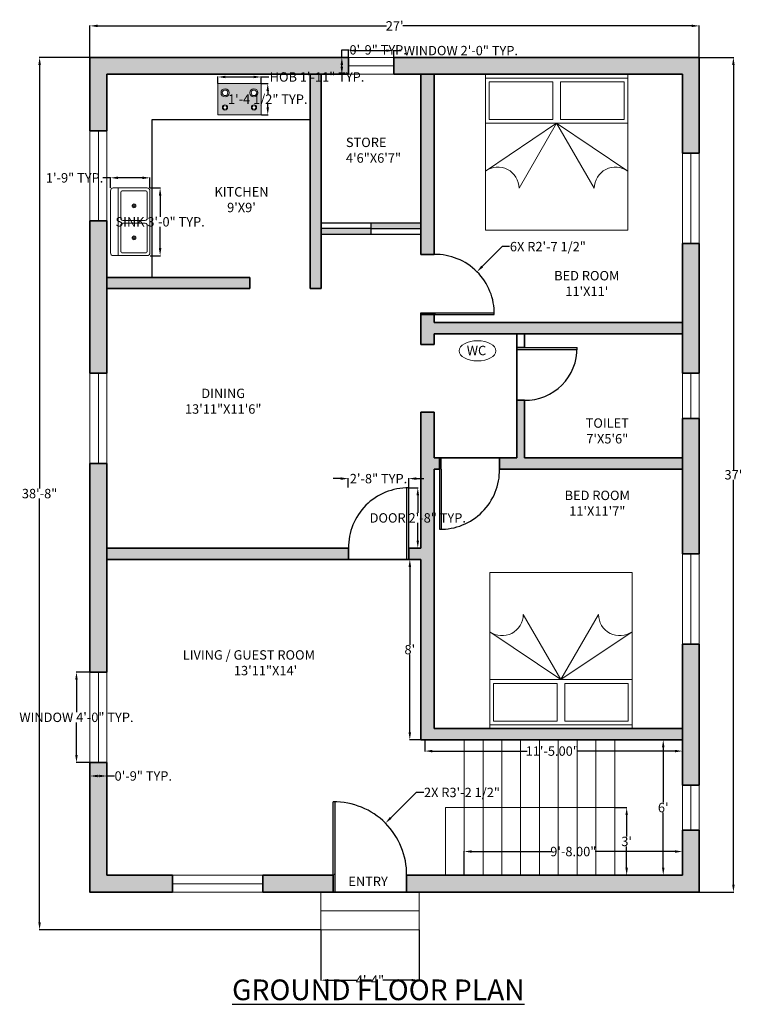
# Model space of a CAD drawing. Units: inches. Extents: x 107756 to 108945, y 133180 to 133782.
# Tile 2 of 3: x 108116 to 108500, y 133209 to 133733. Entities that reach past the tile are written whole.
import ezdxf

# ---------------------------------------------------------------- set-up
doc = ezdxf.new("R2010")
doc.units = ezdxf.units.IN
for name, color, linetype, lineweight in [('A-ANNO-DIMS', 2, 'Continuous', 13), ('A-ANNO-TEXT', 7, 'Continuous', 25), ('A-AREA-IDEN', 7, 'Continuous', 18), ('A-CASE', 8, 'Continuous', 25), ('A-DOOR', 3, 'Continuous', 25), ('A-DOOR-PATT', 7, 'Continuous', 13), ('A-EQPM', 8, 'Continuous', 18), ('A-FLOR-FIXT', 9, 'Continuous', 18), ('A-FLOR-STRS', 7, 'Continuous', 18), ('A-FURN', 8, 'Continuous', 18), ('A-GLAZ', 5, 'Continuous', 18), ('A-WALL', 7, 'Continuous', 35), ('A-WALL-PATT', 252, 'Continuous', 13)]:
    doc.layers.add(name, color=color, linetype=linetype, lineweight=lineweight)
doc.styles.get("Standard").update_dxf_attribs({"font": 'arial.ttf', "height": 5})
doc.styles.add('style1', font='arial.ttf', dxfattribs={"height": 11})
doc.dimstyles.get("Standard").update_dxf_attribs({"dimtxt": 5, "dimasz": 4, "dimexe": 0.18, "dimexo": 0.0625, "dimgap": 0.09, "dimtad": 0, "dimtih": 1, "dimtoh": 1, "dimzin": 0, "dimdsep": 46, "dimlunit": 3, "dimtxsty": 'Standard', "dimcen": 0.09, "dimclrd": 7, "dimclre": 256, "dimclrt": 256, "dimadec": 0, "dimazin": 0, "dimtfac": 1, "dimtofl": 0, "dimtmove": 0, "dimatfit": 3, "dimfxl": 1, "dimtolj": 1, "dimtzin": 0, "dimarcsym": 0})

# ---------------------------------------------------------------- blocks, each defined once
blk = doc.blocks.new('*D22')
at = {"layer": 'A-ANNO-DIMS', "color": 0, "lineweight": -2, "transparency": 16777216}
for p, q in [((108331.1, 133349.82), (108331.1, 133343.75)), ((108468.1, 133349.82), (108468.1, 133343.75)), ((108335.1, 133343.93), (108385.61, 133343.93)), ((108464.1, 133343.93), (108412.2, 133343.93))]:
    blk.add_line(p, q, dxfattribs=at)
at = {"layer": 'A-ANNO-DIMS', "color": 0, "transparency": 16777216}
for points in [[(108335.1, 133344.6), (108335.1, 133343.26), (108331.1, 133343.93)], [(108464.1, 133344.6), (108464.1, 133343.26), (108468.1, 133343.93)]]:
    blk.add_solid(points, dxfattribs=at)
at = {"layer": 'Defpoints', "color": 0, "transparency": 16777216}
for p in [(108331.1, 133349.89), (108468.1, 133349.89), (108331.1, 133343.93)]:
    blk.add_point(p, dxfattribs=at)
at = {"layer": 'A-ANNO-DIMS', "color": 0, "transparency": 16777216, "insert": (108398.9, 133343.93), "char_height": 5, "attachment_point": 5}
blk.add_mtext('\\A1;11\'-5.00"', dxfattribs=at)
blk = doc.blocks.new('*D23')
at = {"layer": 'A-ANNO-DIMS', "color": 0, "lineweight": -2, "transparency": 16777216}
for p, q in [((108352.1, 133277.95), (108352.1, 133290.69)), ((108356.1, 133290.51), (108398.51, 133290.51)), ((108464.1, 133290.51), (108421.69, 133290.51)), ((108468.1, 133277.95), (108468.1, 133290.69))]:
    blk.add_line(p, q, dxfattribs=at)
at = {"layer": 'A-ANNO-DIMS', "color": 0, "transparency": 16777216}
for points in [[(108356.1, 133291.18), (108356.1, 133289.84), (108352.1, 133290.51)], [(108464.1, 133291.18), (108464.1, 133289.84), (108468.1, 133290.51)]]:
    blk.add_solid(points, dxfattribs=at)
at = {"layer": 'Defpoints', "color": 0, "transparency": 16777216}
for p in [(108468.1, 133290.51), (108352.1, 133277.89), (108468.1, 133277.89)]:
    blk.add_point(p, dxfattribs=at)
at = {"layer": 'A-ANNO-DIMS', "color": 0, "transparency": 16777216, "insert": (108410.1, 133290.51), "char_height": 5, "attachment_point": 5}
blk.add_mtext('\\A1;9\'-8.00"', dxfattribs=at)
blk = doc.blocks.new('*D24')
at = {"layer": 'A-ANNO-DIMS', "color": 0, "lineweight": -2, "transparency": 16777216}
for p, q in [((108432.16, 133313.89), (108438.64, 133313.89)), ((108438.46, 133309.89), (108438.46, 133298.53)), ((108438.46, 133281.89), (108438.46, 133293.24)), ((108432.16, 133277.89), (108438.64, 133277.89))]:
    blk.add_line(p, q, dxfattribs=at)
at = {"layer": 'A-ANNO-DIMS', "color": 0, "transparency": 16777216}
for points in [[(108437.8, 133309.89), (108439.13, 133309.89), (108438.46, 133313.89)], [(108437.8, 133281.89), (108439.13, 133281.89), (108438.46, 133277.89)]]:
    blk.add_solid(points, dxfattribs=at)
at = {"layer": 'Defpoints', "color": 0, "transparency": 16777216}
for p in [(108432.1, 133313.89), (108438.46, 133313.89), (108432.1, 133277.89)]:
    blk.add_point(p, dxfattribs=at)
at = {"layer": 'A-ANNO-DIMS', "color": 0, "transparency": 16777216, "insert": (108438.46, 133295.89), "char_height": 5, "attachment_point": 5}
blk.add_mtext("\\A1;3'", dxfattribs=at)
blk = doc.blocks.new('*D25')
at = {"layer": 'A-ANNO-DIMS', "color": 0, "lineweight": -2, "transparency": 16777216}
for p, q in [((108468.04, 133349.89), (108457.74, 133349.89)), ((108457.92, 133345.89), (108457.92, 133316.53)), ((108457.92, 133281.89), (108457.92, 133311.24)), ((108468.04, 133277.89), (108457.74, 133277.89))]:
    blk.add_line(p, q, dxfattribs=at)
at = {"layer": 'A-ANNO-DIMS', "color": 0, "transparency": 16777216}
for points in [[(108457.25, 133345.89), (108458.58, 133345.89), (108457.92, 133349.89)], [(108457.25, 133281.89), (108458.58, 133281.89), (108457.92, 133277.89)]]:
    blk.add_solid(points, dxfattribs=at)
at = {"layer": 'Defpoints', "color": 0, "transparency": 16777216}
for p in [(108457.92, 133349.89), (108468.1, 133349.89), (108468.1, 133277.89)]:
    blk.add_point(p, dxfattribs=at)
at = {"layer": 'A-ANNO-DIMS', "color": 0, "transparency": 16777216, "insert": (108457.92, 133313.89), "char_height": 5, "attachment_point": 5}
blk.add_mtext("\\A1;6'", dxfattribs=at)
blk = doc.blocks.new('*D26')
at = {"layer": 'A-ANNO-DIMS', "color": 0, "lineweight": -2, "transparency": 16777216}
for p, q in [((108329.04, 133445.89), (108322.98, 133445.89)), ((108323.16, 133441.89), (108323.16, 133400.53)), ((108323.16, 133353.89), (108323.16, 133395.24)), ((108329.04, 133349.89), (108322.98, 133349.89))]:
    blk.add_line(p, q, dxfattribs=at)
at = {"layer": 'A-ANNO-DIMS', "color": 0, "transparency": 16777216}
for points in [[(108322.49, 133441.89), (108323.83, 133441.89), (108323.16, 133445.89)], [(108322.49, 133353.89), (108323.83, 133353.89), (108323.16, 133349.89)]]:
    blk.add_solid(points, dxfattribs=at)
at = {"layer": 'Defpoints', "color": 0, "transparency": 16777216}
for p in [(108323.16, 133445.89), (108329.1, 133445.89), (108329.1, 133349.89)]:
    blk.add_point(p, dxfattribs=at)
at = {"layer": 'A-ANNO-DIMS', "color": 0, "transparency": 16777216, "insert": (108323.16, 133397.89), "char_height": 5, "attachment_point": 5}
blk.add_mtext("\\A1;8'", dxfattribs=at)
blk = doc.blocks.new('NEW BED')
for p, q in [((-75.7, 82.92), (0, 82.92)), ((-75.7, 0), (-75.7, 82.92)), ((-75.7, 80.92), (0, 80.92)), ((-73.7, 78.92), (-39.85, 78.92)), ((-73.7, 58.92), (-73.7, 78.92)), ((-39.85, 58.92), (-39.85, 78.92)), ((-35.85, 78.92), (-2, 78.92)), ((-35.85, 58.92), (-35.85, 78.92)), ((-2, 78.92), (-2, 58.92)), ((0, 82.92), (0, 0)), ((-73.7, 58.92), (-39.85, 58.92)), ((-35.85, 58.92), (-2, 58.92)), ((-75.7, 56.92), (0, 56.92)), ((-37.85, 56.92), (-75.7, 31.45)), ((-37.85, 56.92), (-57.85, 22.27)), ((-37.85, 56.92), (0, 31.45)), ((-37.85, 56.92), (-17.84, 22.27)), ((0, 0), (-75.7, 0))]:
    blk.add_line(p, q)
for centre, start, end in [((-69.14, 22.27), 0, 125.5497), ((-6.56, 22.27), 54.4503, 180)]:
    blk.add_arc(centre, 11.28, start, end)
blk = doc.blocks.new('stov')
h = blk.add_hatch(color=256)
h.dxf.hatch_style = 1
h.set_gradient(color1=(255, 255, 255), color2=(147, 149, 152), name='CYLINDER')
h.paths.add_polyline_path([(0, 0), (16.67, 0), (16.67, 23.1), (0, 23.1)])
h.paths.add_polyline_path([(2.78, 19.21, -1), (7.12, 19.21, -1)], flags=16)
h.paths.add_polyline_path([(3.47, 19.21, -1), (6.43, 19.21, -1)], flags=0)
h.paths.add_polyline_path([(7.12, 3.89, -1), (2.78, 3.89, -1)], flags=16)
h.paths.add_polyline_path([(6.43, 3.89, -1), (3.47, 3.89, -1)], flags=0)
h.paths.add_polyline_path([(11.35, 19.27, -1), (14.15, 19.27, -1)], flags=16)
h.paths.add_polyline_path([(11.81, 19.27, -1), (13.68, 19.27, -1)], flags=0)
h.paths.add_polyline_path([(14.15, 3.83, -1), (11.35, 3.83, -1)], flags=16)
blk.add_lwpolyline([(16.67, 0), (0, 0), (0, 23.1), (16.67, 23.1)], close=True)
for centre, radius in [((4.95, 19.21), 2.17), ((4.95, 19.21), 2.17), ((4.95, 19.21), 1.48), ((12.75, 19.27), 1.4), ((12.75, 19.27), 0.936), ((4.95, 3.89), 2.17), ((4.95, 3.89), 2.17), ((4.95, 3.89), 1.48), ((12.75, 3.83), 1.4), ((12.75, 3.83), 0.936)]:
    blk.add_circle(centre, radius)
blk = doc.blocks.new('Sink-double - 36 in top')
for p, q in [((-18, -4), (18, -4)), ((-0.75, -18.5), (-0.75, -6.5)), ((0.75, -6.5), (0.75, -18.5))]:
    blk.add_line(p, q)
for points in [[(-16.5, 0), (16.5, 0)], [(-18, -19.5), (-18, -1.5)], [(18, -1.5), (18, -19.5)], [(-16.5, -18.5), (-16.5, -6.5)], [(-15.5, -5.5), (-1.75, -5.5)], [(1.75, -5.5), (15.5, -5.5)], [(16.5, -6.5), (16.5, -18.5)], [(-1.75, -19.5), (-15.5, -19.5)], [(15.5, -19.5), (1.75, -19.5)], [(16.5, -21), (-16.5, -21)]]:
    blk.add_lwpolyline(points)
for centre, radius in [((-8.5, -12.5), 1), ((-8.5, -12.5), 0.5), ((8.5, -12.5), 1), ((8.5, -12.5), 0.5)]:
    blk.add_circle(centre, radius)
for centre, radius, start, end in [((-16.5, -1.5), 1.5, 90, 180), ((16.5, -1.5), 1.5, 0, 90), ((-15.5, -6.5), 1, 90, 180), ((-1.75, -6.5), 1, 0, 90), ((1.75, -6.5), 1, 90, 180), ((15.5, -6.5), 1, 0, 90), ((-16.5, -19.5), 1.5, 180, 270), ((-15.5, -18.5), 1, 180, 270), ((-1.75, -18.5), 1, 270, 0), ((1.75, -18.5), 1, 180, 270), ((15.5, -18.5), 1, 270, 0), ((16.5, -19.5), 1.5, 270, 0)]:
    blk.add_arc(centre, radius, start, end)
blk = doc.blocks.new('*D30')
at = {"layer": 'A-ANNO-DIMS', "color": 0, "lineweight": -2, "transparency": 16777216}
for p, q in [((108153.1, 133712.95), (108153.1, 133729.82)), ((108157.1, 133729.64), (108310.72, 133729.64)), ((108473.1, 133729.64), (108319.47, 133729.64)), ((108477.1, 133712.95), (108477.1, 133729.82))]:
    blk.add_line(p, q, dxfattribs=at)
at = {"layer": 'A-ANNO-DIMS', "color": 0, "transparency": 16777216}
for points in [[(108157.1, 133730.31), (108157.1, 133728.98), (108153.1, 133729.64)], [(108473.1, 133730.31), (108473.1, 133728.98), (108477.1, 133729.64)]]:
    blk.add_solid(points, dxfattribs=at)
at = {"layer": 'Defpoints', "color": 0, "transparency": 16777216}
for p in [(108477.1, 133729.64), (108153.1, 133712.89), (108477.1, 133712.89)]:
    blk.add_point(p, dxfattribs=at)
at = {"layer": 'A-ANNO-DIMS', "color": 0, "transparency": 16777216, "insert": (108315.1, 133729.64), "char_height": 5, "attachment_point": 5}
blk.add_mtext("\\A1;27'", dxfattribs=at)
blk = doc.blocks.new('*D31')
at = {"layer": 'A-ANNO-DIMS', "color": 0, "lineweight": -2, "transparency": 16777216}
for p, q in [((108477.16, 133712.89), (108495.4, 133712.89)), ((108495.22, 133708.89), (108495.22, 133493.53)), ((108495.22, 133272.89), (108495.22, 133488.24)), ((108477.16, 133268.89), (108495.4, 133268.89))]:
    blk.add_line(p, q, dxfattribs=at)
at = {"layer": 'A-ANNO-DIMS', "color": 0, "transparency": 16777216}
for points in [[(108494.56, 133708.89), (108495.89, 133708.89), (108495.22, 133712.89)], [(108494.56, 133272.89), (108495.89, 133272.89), (108495.22, 133268.89)]]:
    blk.add_solid(points, dxfattribs=at)
at = {"layer": 'Defpoints', "color": 0, "transparency": 16777216}
for p in [(108477.1, 133712.89), (108477.1, 133268.89), (108495.22, 133268.89)]:
    blk.add_point(p, dxfattribs=at)
at = {"layer": 'A-ANNO-DIMS', "color": 0, "transparency": 16777216, "insert": (108495.22, 133490.89), "char_height": 5, "attachment_point": 5}
blk.add_mtext("\\A1;37'", dxfattribs=at)
blk = doc.blocks.new('DOOR-SWING-28IN')
for p, q in [((0, 28), (28, 28)), ((0, 27), (28, 27))]:
    blk.add_line(p, q)
blk.add_arc((0.5, 27.5), 27.5, 268.9584, 1.0416)
blk = doc.blocks.new('DOOR-SWING-32IN')
for p, q in [((0, 1), (32, 1)), ((0, 0), (32, 0))]:
    blk.add_line(p, q)
blk.add_arc((0.5, 0.5), 31.5, 359.0906, 90.9094)
blk = doc.blocks.new('DOOR-SWING-39IN')
for p, q in [((0, 0), (0, 39)), ((1, 0), (1, 39))]:
    blk.add_line(p, q)
blk.add_arc((0.5, 0.5), 38.5, 359.2559, 90.7441)
blk = doc.blocks.new('WIN-48IN')
blk.add_line((48, 4.5), (0, 4.5))
blk.add_lwpolyline([(0, 0), (48, 0), (48, 9), (0, 9)], close=True)
blk = doc.blocks.new('WIN-24IN')
blk.add_line((0, 4.5), (24, 4.5))
blk.add_lwpolyline([(0, 9), (24, 9), (24, 0), (0, 0)], close=True)
blk = doc.blocks.new('*D49')
at = {"layer": 'A-ANNO-DIMS', "lineweight": -2, "transparency": 16777216}
for p, q in [((108153.04, 133385.89), (108145.72, 133385.89)), ((108153.04, 133337.89), (108145.72, 133337.89))]:
    blk.add_line(p, q, dxfattribs=at)
at = {"layer": 'A-ANNO-DIMS', "color": 7, "lineweight": -2, "transparency": 16777216}
for p, q in [((108145.9, 133381.89), (108145.9, 133364.56)), ((108145.9, 133341.89), (108145.9, 133359.21))]:
    blk.add_line(p, q, dxfattribs=at)
at = {"layer": 'A-ANNO-DIMS', "color": 7, "transparency": 16777216}
for points in [[(108145.23, 133381.89), (108146.57, 133381.89), (108145.9, 133385.89)], [(108145.23, 133341.89), (108146.57, 133341.89), (108145.9, 133337.89)]]:
    blk.add_solid(points, dxfattribs=at)
at = {"layer": 'Defpoints', "color": 0, "transparency": 16777216}
for p in [(108153.1, 133385.89), (108145.9, 133337.89), (108153.1, 133337.89)]:
    blk.add_point(p, dxfattribs=at)
at = {"layer": 'A-ANNO-DIMS', "transparency": 16777216, "insert": (108145.9, 133361.89), "char_height": 5, "attachment_point": 5}
blk.add_mtext('\\A1;WINDOW 4\'-0" TYP.', dxfattribs=at)
blk = doc.blocks.new('*D50')
at = {"layer": 'A-ANNO-DIMS', "lineweight": -2, "transparency": 16777216}
for p, q in [((108153.1, 133337.82), (108153.1, 133330.51)), ((108162.1, 133337.82), (108162.1, 133330.51))]:
    blk.add_line(p, q, dxfattribs=at)
at = {"layer": 'A-ANNO-DIMS', "color": 7, "lineweight": -2, "transparency": 16777216}
for p, q in [((108157.1, 133330.69), (108158.1, 133330.69)), ((108162.1, 133330.69), (108166.1, 133330.69))]:
    blk.add_line(p, q, dxfattribs=at)
at = {"layer": 'A-ANNO-DIMS', "color": 7, "transparency": 16777216}
for points in [[(108157.1, 133331.35), (108157.1, 133330.02), (108153.1, 133330.69)], [(108158.1, 133331.35), (108158.1, 133330.02), (108162.1, 133330.69)]]:
    blk.add_solid(points, dxfattribs=at)
at = {"layer": 'Defpoints', "color": 0, "transparency": 16777216}
for p in [(108153.1, 133337.89), (108162.1, 133337.89), (108162.1, 133330.69)]:
    blk.add_point(p, dxfattribs=at)
at = {"layer": 'A-ANNO-DIMS', "transparency": 16777216, "insert": (108181.43, 133330.69), "char_height": 5, "attachment_point": 5}
blk.add_mtext('\\A1;0\'-9" TYP.', dxfattribs=at)
blk = doc.blocks.new('*D51')
at = {"layer": 'A-ANNO-DIMS', "lineweight": -2, "transparency": 16777216}
for p, q in [((108290.6, 133712.95), (108290.6, 133716.67)), ((108314.6, 133712.95), (108314.6, 133716.67))]:
    blk.add_line(p, q, dxfattribs=at)
at = {"layer": 'A-ANNO-DIMS', "color": 7, "lineweight": -2, "transparency": 16777216}
for p, q in [((108294.6, 133716.49), (108310.6, 133716.49)), ((108314.6, 133716.49), (108318.6, 133716.49))]:
    blk.add_line(p, q, dxfattribs=at)
at = {"layer": 'A-ANNO-DIMS', "color": 7, "transparency": 16777216}
for points in [[(108294.6, 133717.15), (108294.6, 133715.82), (108290.6, 133716.49)], [(108310.6, 133717.15), (108310.6, 133715.82), (108314.6, 133716.49)]]:
    blk.add_solid(points, dxfattribs=at)
at = {"layer": 'Defpoints', "color": 0, "transparency": 16777216}
for p in [(108314.6, 133716.49), (108290.6, 133712.89), (108314.6, 133712.89)]:
    blk.add_point(p, dxfattribs=at)
at = {"layer": 'A-ANNO-DIMS', "transparency": 16777216, "insert": (108350.32, 133716.49), "char_height": 5, "attachment_point": 5}
blk.add_mtext('\\A1;WINDOW 2\'-0" TYP.', dxfattribs=at)
blk = doc.blocks.new('*D52')
at = {"layer": 'A-ANNO-DIMS', "color": 7, "lineweight": -2, "transparency": 16777216}
for p, q in [((108287, 133712.89), (108287, 133716.89)), ((108287, 133716.89), (108291, 133716.89)), ((108287, 133707.89), (108287, 133708.89))]:
    blk.add_line(p, q, dxfattribs=at)
at = {"layer": 'A-ANNO-DIMS', "lineweight": -2, "transparency": 16777216}
for p, q in [((108290.54, 133712.89), (108286.82, 133712.89)), ((108290.54, 133703.89), (108286.82, 133703.89))]:
    blk.add_line(p, q, dxfattribs=at)
at = {"layer": 'A-ANNO-DIMS', "color": 7, "transparency": 16777216}
for points in [[(108286.33, 133708.89), (108287.67, 133708.89), (108287, 133712.89)], [(108286.33, 133707.89), (108287.67, 133707.89), (108287, 133703.89)]]:
    blk.add_solid(points, dxfattribs=at)
at = {"layer": 'Defpoints', "color": 0, "transparency": 16777216}
for p in [(108287, 133712.89), (108290.6, 133712.89), (108290.6, 133703.89)]:
    blk.add_point(p, dxfattribs=at)
at = {"layer": 'A-ANNO-DIMS', "transparency": 16777216, "insert": (108306.33, 133716.89), "char_height": 5, "attachment_point": 5}
blk.add_mtext('\\A1;0\'-9" TYP.', dxfattribs=at)
blk = doc.blocks.new('*D53')
at = {"layer": 'A-ANNO-DIMS', "lineweight": -2, "transparency": 16777216}
for p, q in [((108322.64, 133484.02), (108327.58, 133484.02)), ((108322.64, 133451.89), (108327.58, 133451.89))]:
    blk.add_line(p, q, dxfattribs=at)
at = {"layer": 'A-ANNO-DIMS', "color": 7, "lineweight": -2, "transparency": 16777216}
for p, q in [((108327.4, 133480.02), (108327.4, 133470.63)), ((108327.4, 133455.89), (108327.4, 133465.28))]:
    blk.add_line(p, q, dxfattribs=at)
at = {"layer": 'A-ANNO-DIMS', "color": 7, "transparency": 16777216}
for points in [[(108326.73, 133480.02), (108328.06, 133480.02), (108327.4, 133484.02)], [(108326.73, 133455.89), (108328.06, 133455.89), (108327.4, 133451.89)]]:
    blk.add_solid(points, dxfattribs=at)
at = {"layer": 'Defpoints', "color": 0, "transparency": 16777216}
for p in [(108322.58, 133484.02), (108327.4, 133484.02), (108322.58, 133451.89)]:
    blk.add_point(p, dxfattribs=at)
at = {"layer": 'A-ANNO-DIMS', "transparency": 16777216, "insert": (108327.4, 133467.95), "char_height": 5, "attachment_point": 5}
blk.add_mtext('\\A1;DOOR 2\'-8" TYP.', dxfattribs=at)
blk = doc.blocks.new('*D54')
at = {"layer": 'A-ANNO-DIMS', "color": 7, "lineweight": -2, "transparency": 16777216}
for p, q in [((108286.44, 133488.84), (108282.44, 133488.84)), ((108326.58, 133488.84), (108330.58, 133488.84))]:
    blk.add_line(p, q, dxfattribs=at)
at = {"layer": 'A-ANNO-DIMS', "lineweight": -2, "transparency": 16777216}
for p, q in [((108290.44, 133484.08), (108290.44, 133489.02)), ((108322.58, 133484.08), (108322.58, 133489.02))]:
    blk.add_line(p, q, dxfattribs=at)
at = {"layer": 'A-ANNO-DIMS', "color": 7, "transparency": 16777216}
for points in [[(108286.44, 133489.51), (108286.44, 133488.18), (108290.44, 133488.84)], [(108326.58, 133489.51), (108326.58, 133488.18), (108322.58, 133488.84)]]:
    blk.add_solid(points, dxfattribs=at)
at = {"layer": 'Defpoints', "color": 0, "transparency": 16777216}
for p in [(108290.44, 133488.84), (108290.44, 133484.02), (108322.58, 133484.02)]:
    blk.add_point(p, dxfattribs=at)
at = {"layer": 'A-ANNO-DIMS', "transparency": 16777216, "insert": (108306.51, 133488.84), "char_height": 5, "attachment_point": 5}
blk.add_mtext('\\A1;2\'-8" TYP.', dxfattribs=at)
blk = doc.blocks.new('*D61')
at = {"layer": 'A-ANNO-DIMS', "lineweight": -2, "transparency": 16777216}
for p, q in [((108221.05, 133699.06), (108221.05, 133702.65)), ((108244.15, 133699.06), (108244.15, 133702.65))]:
    blk.add_line(p, q, dxfattribs=at)
at = {"layer": 'A-ANNO-DIMS', "color": 7, "lineweight": -2, "transparency": 16777216}
for p, q in [((108225.05, 133702.47), (108240.15, 133702.47)), ((108244.15, 133702.47), (108248.15, 133702.47))]:
    blk.add_line(p, q, dxfattribs=at)
at = {"layer": 'A-ANNO-DIMS', "color": 7, "transparency": 16777216}
for points in [[(108225.05, 133703.13), (108225.05, 133701.8), (108221.05, 133702.47)], [(108240.15, 133703.13), (108240.15, 133701.8), (108244.15, 133702.47)]]:
    blk.add_solid(points, dxfattribs=at)
at = {"layer": 'Defpoints', "color": 0, "transparency": 16777216}
for p in [(108221.05, 133699), (108244.15, 133702.47), (108244.15, 133699)]:
    blk.add_point(p, dxfattribs=at)
at = {"layer": 'A-ANNO-DIMS', "transparency": 16777216, "insert": (108273.82, 133702.47), "char_height": 5, "attachment_point": 5}
blk.add_mtext('\\A1;HOB 1\'-11" TYP.', dxfattribs=at)
blk = doc.blocks.new('*D62')
at = {"layer": 'A-ANNO-DIMS', "lineweight": -2, "transparency": 16777216}
for p, q in [((108244.21, 133699), (108247.79, 133699)), ((108244.21, 133682.33), (108247.79, 133682.33))]:
    blk.add_line(p, q, dxfattribs=at)
at = {"layer": 'A-ANNO-DIMS', "color": 7, "lineweight": -2, "transparency": 16777216}
for p, q in [((108247.61, 133695), (108247.61, 133693.34)), ((108247.61, 133686.33), (108247.61, 133687.99))]:
    blk.add_line(p, q, dxfattribs=at)
at = {"layer": 'A-ANNO-DIMS', "color": 7, "transparency": 16777216}
for points in [[(108246.94, 133695), (108248.28, 133695), (108247.61, 133699)], [(108246.94, 133686.33), (108248.28, 133686.33), (108247.61, 133682.33)]]:
    blk.add_solid(points, dxfattribs=at)
at = {"layer": 'Defpoints', "color": 0, "transparency": 16777216}
for p in [(108244.15, 133699), (108244.15, 133682.33), (108247.61, 133682.33)]:
    blk.add_point(p, dxfattribs=at)
at = {"layer": 'A-ANNO-DIMS', "transparency": 16777216, "insert": (108247.61, 133690.66), "char_height": 5, "attachment_point": 5}
blk.add_mtext('\\A1;1\'-4 1/2" TYP.', dxfattribs=at)
blk = doc.blocks.new('*D63')
at = {"layer": 'A-ANNO-DIMS', "lineweight": -2, "transparency": 16777216}
for p, q in [((108185.06, 133643.42), (108190.57, 133643.42)), ((108185.06, 133607.42), (108190.57, 133607.42))]:
    blk.add_line(p, q, dxfattribs=at)
at = {"layer": 'A-ANNO-DIMS', "color": 7, "lineweight": -2, "transparency": 16777216}
for p, q in [((108190.39, 133639.42), (108190.39, 133628.1)), ((108190.39, 133611.42), (108190.39, 133622.75))]:
    blk.add_line(p, q, dxfattribs=at)
at = {"layer": 'A-ANNO-DIMS', "color": 7, "transparency": 16777216}
for points in [[(108189.73, 133639.42), (108191.06, 133639.42), (108190.39, 133643.42)], [(108189.73, 133611.42), (108191.06, 133611.42), (108190.39, 133607.42)]]:
    blk.add_solid(points, dxfattribs=at)
at = {"layer": 'Defpoints', "color": 0, "transparency": 16777216}
for p in [(108184.99, 133643.42), (108190.39, 133643.42), (108184.99, 133607.42)]:
    blk.add_point(p, dxfattribs=at)
at = {"layer": 'A-ANNO-DIMS', "transparency": 16777216, "insert": (108190.39, 133625.42), "char_height": 5, "attachment_point": 5}
blk.add_mtext('\\A1;SINK 3\'-0" TYP.', dxfattribs=at)
blk = doc.blocks.new('*D64')
at = {"layer": 'A-ANNO-DIMS', "color": 7, "lineweight": -2, "transparency": 16777216}
for p, q in [((108163.99, 133648.82), (108159.99, 133648.82)), ((108180.99, 133648.82), (108167.99, 133648.82))]:
    blk.add_line(p, q, dxfattribs=at)
at = {"layer": 'A-ANNO-DIMS', "lineweight": -2, "transparency": 16777216}
for p, q in [((108163.99, 133643.49), (108163.99, 133649)), ((108184.99, 133643.49), (108184.99, 133649))]:
    blk.add_line(p, q, dxfattribs=at)
at = {"layer": 'A-ANNO-DIMS', "color": 7, "transparency": 16777216}
for points in [[(108167.99, 133649.49), (108167.99, 133648.16), (108163.99, 133648.82)], [(108180.99, 133649.49), (108180.99, 133648.16), (108184.99, 133648.82)]]:
    blk.add_solid(points, dxfattribs=at)
at = {"layer": 'Defpoints', "color": 0, "transparency": 16777216}
for p in [(108163.99, 133648.82), (108163.99, 133643.42), (108184.99, 133643.42)]:
    blk.add_point(p, dxfattribs=at)
at = {"layer": 'A-ANNO-DIMS', "transparency": 16777216, "insert": (108144.9, 133648.82), "char_height": 5, "attachment_point": 5}
blk.add_mtext('\\A1;1\'-9" TYP.', dxfattribs=at)
blk = doc.blocks.new('*D65')
at = {"layer": 'A-ANNO-DIMS', "lineweight": -2, "transparency": 16777216}
for p, q in [((108275.87, 133248.82), (108275.87, 133221.91)), ((108328.06, 133248.82), (108328.06, 133221.91))]:
    blk.add_line(p, q, dxfattribs=at)
at = {"layer": 'A-ANNO-DIMS', "color": 7, "lineweight": -2, "transparency": 16777216}
for p, q in [((108279.87, 133222.09), (108295.13, 133222.09)), ((108324.06, 133222.09), (108308.8, 133222.09))]:
    blk.add_line(p, q, dxfattribs=at)
at = {"layer": 'A-ANNO-DIMS', "color": 7, "transparency": 16777216}
for points in [[(108279.87, 133222.75), (108279.87, 133221.42), (108275.87, 133222.09)], [(108324.06, 133222.75), (108324.06, 133221.42), (108328.06, 133222.09)]]:
    blk.add_solid(points, dxfattribs=at)
at = {"layer": 'Defpoints', "color": 0, "transparency": 16777216}
for p in [(108275.87, 133248.89), (108328.06, 133248.89), (108328.06, 133222.09)]:
    blk.add_point(p, dxfattribs=at)
at = {"layer": 'A-ANNO-DIMS', "transparency": 16777216, "insert": (108301.96, 133222.09), "char_height": 5, "attachment_point": 5}
blk.add_mtext('\\A1;4\'-4"', dxfattribs=at)
blk = doc.blocks.new('*D66')
at = {"layer": 'A-ANNO-DIMS', "lineweight": -2, "transparency": 16777216}
for p, q in [((108153.04, 133712.89), (108126.12, 133712.89)), ((108275.8, 133248.89), (108126.12, 133248.89))]:
    blk.add_line(p, q, dxfattribs=at)
at = {"layer": 'A-ANNO-DIMS', "color": 7, "lineweight": -2, "transparency": 16777216}
for p, q in [((108126.3, 133708.89), (108126.3, 133483.53)), ((108126.3, 133252.89), (108126.3, 133478.24))]:
    blk.add_line(p, q, dxfattribs=at)
at = {"layer": 'A-ANNO-DIMS', "color": 7, "transparency": 16777216}
for points in [[(108125.63, 133708.89), (108126.97, 133708.89), (108126.3, 133712.89)], [(108125.63, 133252.89), (108126.97, 133252.89), (108126.3, 133248.89)]]:
    blk.add_solid(points, dxfattribs=at)
at = {"layer": 'Defpoints', "color": 0, "transparency": 16777216}
for p in [(108153.1, 133712.89), (108126.3, 133248.89), (108275.87, 133248.89)]:
    blk.add_point(p, dxfattribs=at)
at = {"layer": 'A-ANNO-DIMS', "transparency": 16777216, "insert": (108126.3, 133480.89), "char_height": 5, "attachment_point": 5}
blk.add_mtext('\\A1;38\'-8"', dxfattribs=at)
blk = doc.blocks.new('*D67')
at = {"layer": 'A-ANNO-DIMS', "color": 7, "lineweight": -2, "transparency": 16777216}
for p, q in [((108326.53, 133321.95), (108313.02, 133308.44)), ((108330.53, 133321.95), (108326.53, 133321.95))]:
    blk.add_line(p, q, dxfattribs=at)
at = {"layer": 'A-ANNO-DIMS', "lineweight": -2, "transparency": 16777216}
for p, q in [((108282.87, 133278.39), (108283.05, 133278.39)), ((108282.96, 133278.3), (108282.96, 133278.48))]:
    blk.add_line(p, q, dxfattribs=at)
at = {"layer": 'A-ANNO-DIMS', "color": 7, "transparency": 16777216}
blk.add_solid([(108312.55, 133308.91), (108313.49, 133307.97), (108310.19, 133305.61)], dxfattribs=at)
at = {"layer": 'Defpoints', "color": 0, "transparency": 16777216}
for p in [(108310.19, 133305.61), (108282.96, 133278.39)]:
    blk.add_point(p, dxfattribs=at)
at = {"layer": 'A-ANNO-DIMS', "transparency": 16777216, "insert": (108350.89, 133321.95), "char_height": 5, "attachment_point": 5}
blk.add_mtext('\\A1;2X R3\'-2 1/2"', dxfattribs=at)
blk = doc.blocks.new('*D68')
at = {"layer": 'A-ANNO-DIMS', "color": 7, "lineweight": -2, "transparency": 16777216}
for p, q in [((108372.24, 133612.24), (108361.7, 133601.7)), ((108376.24, 133612.24), (108372.24, 133612.24))]:
    blk.add_line(p, q, dxfattribs=at)
at = {"layer": 'A-ANNO-DIMS', "lineweight": -2, "transparency": 16777216}
for p, q in [((108336.51, 133576.6), (108336.69, 133576.6)), ((108336.6, 133576.51), (108336.6, 133576.69))]:
    blk.add_line(p, q, dxfattribs=at)
at = {"layer": 'A-ANNO-DIMS', "color": 7, "transparency": 16777216}
blk.add_solid([(108361.23, 133602.17), (108362.17, 133601.23), (108358.88, 133598.87)], dxfattribs=at)
at = {"layer": 'Defpoints', "color": 0, "transparency": 16777216}
for p in [(108358.88, 133598.87), (108336.6, 133576.6)]:
    blk.add_point(p, dxfattribs=at)
at = {"layer": 'A-ANNO-DIMS', "transparency": 16777216, "insert": (108396.58, 133612.24), "char_height": 5, "attachment_point": 5}
blk.add_mtext('\\A1;6X R2\'-7 1/2"', dxfattribs=at)

msp = doc.modelspace()

# ---------------------------------------------------------------- hatches: boundary and pattern name
at = {"layer": 'A-DOOR-PATT'}
h = msp.add_hatch(color=256, dxfattribs=at)
h.dxf.hatch_style = 1
h.paths.add_polyline_path([(108302.598, 133621.887), (108276.098, 133621.887), (108276.098, 133618.887), (108302.598, 133618.887)])
h.paths.add_polyline_path([(108329.098, 133624.887), (108302.598, 133624.887), (108302.598, 133621.887), (108329.098, 133621.887)])
at = {"layer": 'A-WALL-PATT'}
h = msp.add_hatch(color=256, dxfattribs=at)
h.dxf.hatch_style = 1
h.paths.add_polyline_path([(108290.598, 133712.887), (108153.098, 133712.887), (108153.098, 133673.887), (108162.098, 133673.887), (108162.098, 133703.887), (108290.598, 133703.887)])
h.paths.add_polyline_path([(108477.098, 133712.887), (108314.598, 133712.887), (108314.598, 133703.887), (108468.098, 133703.887), (108468.098, 133661.887), (108477.098, 133661.887)])
h.paths.add_polyline_path([(108477.098, 133613.887), (108468.098, 133613.887), (108468.098, 133544.887), (108477.098, 133544.887)])
h.paths.add_polyline_path([(108468.098, 133571.887), (108336.098, 133571.887), (108336.098, 133576.096), (108329.098, 133576.096), (108329.098, 133560.095), (108336.098, 133560.095), (108336.098, 133565.887), (108468.098, 133565.887)])
h.paths.add_polyline_path([(108336.098, 133703.887), (108329.098, 133703.887), (108329.098, 133608.096), (108336.098, 133608.096)])
h.paths.add_polyline_path([(108276.098, 133703.887), (108270.098, 133703.887), (108270.098, 133589.887), (108276.098, 133589.887)])
h.paths.add_polyline_path([(108238.098, 133595.887), (108162.098, 133595.887), (108162.098, 133589.887), (108238.098, 133589.887)])
h.paths.add_polyline_path([(108162.098, 133625.887), (108153.098, 133625.887), (108153.098, 133544.887), (108162.098, 133544.887)])
h.paths.add_polyline_path([(108162.098, 133496.887), (108153.098, 133496.887), (108153.098, 133385.887), (108162.098, 133385.887)])
h.paths.add_polyline_path([(108290.575, 133451.887), (108162.098, 133451.887), (108162.098, 133445.887), (108290.575, 133445.887)])
h.paths.add_polyline_path([(108336.098, 133493.887), (108338.874, 133493.887), (108338.874, 133499.887), (108336.098, 133499.887), (108336.098, 133524.127), (108329.098, 133524.127), (108329.098, 133451.887), (108322.575, 133451.887), (108322.575, 133445.887), (108329.098, 133445.887), (108329.098, 133349.887), (108468.098, 133349.887), (108468.098, 133355.887), (108336.098, 133355.887)])
h.paths.add_polyline_path([(108468.098, 133499.887), (108384.098, 133499.887), (108384.098, 133530.549), (108380.098, 133530.549), (108380.098, 133499.887), (108370.874, 133499.887), (108370.874, 133493.887), (108468.098, 133493.887)])
h.paths.add_polyline_path([(108477.098, 133520.887), (108468.098, 133520.887), (108468.098, 133448.887), (108477.098, 133448.887)])
h.paths.add_polyline_path([(108477.098, 133400.887), (108468.098, 133400.887), (108468.098, 133325.887), (108477.098, 133325.887)])
h.paths.add_polyline_path([(108477.098, 133301.887), (108468.098, 133301.887), (108468.098, 133277.887), (108321.465, 133277.887), (108321.465, 133268.887), (108477.098, 133268.887)])
h.paths.add_polyline_path([(108162.098, 133337.887), (108153.098, 133337.887), (108153.098, 133268.887), (108197.048, 133268.887), (108197.048, 133277.887), (108162.098, 133277.887)])
h.paths.add_polyline_path([(108282.465, 133277.887), (108245.048, 133277.887), (108245.048, 133268.887), (108282.465, 133268.887)])

# ---------------------------------------------------------------- linework, layer by layer
at = {"layer": 'A-CASE'}
for p, q in [((108186.098, 133679.887), (108270.098, 133679.887)), ((108186.098, 133595.887), (108186.098, 133679.887))]:
    msp.add_line(p, q, dxfattribs=at)
at = {"layer": 'A-DOOR'}
for p, q in [((108276.098, 133624.887), (108329.098, 133624.887)), ((108302.598, 133618.887), (108302.598, 133624.887)), ((108302.598, 133621.887), (108276.098, 133621.887)), ((108302.598, 133621.887), (108329.098, 133621.887)), ((108276.098, 133618.887), (108329.098, 133618.887)), ((108329.098, 133577.096), (108336.098, 133577.096)), ((108380.098, 133557.549), (108384.098, 133557.549)), ((108339.874, 133493.887), (108339.874, 133499.887)), ((108321.575, 133445.887), (108321.575, 133451.887)), ((108283.465, 133268.887), (108283.465, 133277.887))]:
    msp.add_line(p, q, dxfattribs=at)
at = {"layer": 'A-FLOR-FIXT'}
msp.add_ellipse((108359.159, 133556.797), major_axis=(-9.778, 0), ratio=0.5483685, dxfattribs=at)
at = {"layer": 'A-FLOR-STRS'}
for p, q in [((108352.098, 133349.887), (108352.098, 133277.887)), ((108362.098, 133349.887), (108362.098, 133277.887)), ((108372.098, 133349.887), (108372.098, 133277.887)), ((108382.098, 133349.887), (108382.098, 133277.887)), ((108392.098, 133349.887), (108392.098, 133277.887)), ((108402.098, 133349.887), (108402.098, 133277.887)), ((108412.098, 133349.887), (108412.098, 133277.887)), ((108422.098, 133349.887), (108422.098, 133277.887)), ((108432.098, 133349.887), (108432.098, 133277.887)), ((108432.098, 133313.887), (108342.098, 133313.887)), ((108342.098, 133313.887), (108342.098, 133277.887)), ((108275.867, 133268.887), (108275.867, 133248.887)), ((108328.063, 133268.887), (108328.063, 133248.887)), ((108275.867, 133258.887), (108328.063, 133258.887)), ((108275.867, 133248.887), (108275.867, 133248.887)), ((108275.867, 133248.887), (108328.063, 133248.887))]:
    msp.add_line(p, q, dxfattribs=at)
at = {"layer": 'A-WALL'}
for p, q in [((108290.598, 133703.887), (108290.598, 133712.887)), ((108314.598, 133703.887), (108314.598, 133712.887)), ((108162.098, 133703.887), (108290.598, 133703.887)), ((108162.098, 133673.887), (108162.098, 133703.887)), ((108270.098, 133589.887), (108270.098, 133703.887)), ((108276.098, 133589.887), (108276.098, 133703.887)), ((108314.598, 133703.887), (108468.098, 133703.887)), ((108329.098, 133703.887), (108329.098, 133608.096)), ((108336.098, 133703.887), (108336.098, 133608.096)), ((108468.098, 133703.887), (108468.098, 133661.887)), ((108162.098, 133673.887), (108153.098, 133673.887)), ((108468.098, 133661.887), (108477.098, 133661.887)), ((108162.098, 133625.887), (108153.098, 133625.887)), ((108162.098, 133544.887), (108162.098, 133625.887)), ((108468.098, 133613.887), (108477.098, 133613.887)), ((108468.098, 133613.887), (108468.098, 133544.887)), ((108329.098, 133608.096), (108336.098, 133608.096)), ((108162.098, 133595.887), (108238.098, 133595.887)), ((108238.098, 133589.887), (108238.098, 133595.887)), ((108162.098, 133589.887), (108238.098, 133589.887)), ((108270.098, 133589.887), (108276.098, 133589.887)), ((108329.098, 133577.096), (108329.098, 133560.095)), ((108329.098, 133576.096), (108336.098, 133576.096)), ((108336.098, 133576.096), (108336.098, 133571.887)), ((108336.098, 133571.887), (108468.098, 133571.887)), ((108336.098, 133565.887), (108468.098, 133565.887)), ((108336.098, 133565.887), (108336.098, 133560.095)), ((108380.098, 133565.887), (108380.098, 133499.887)), ((108384.098, 133565.887), (108384.098, 133558.549)), ((108336.098, 133560.095), (108329.098, 133560.095)), ((108380.098, 133558.549), (108384.098, 133558.549)), ((108162.098, 133544.887), (108153.098, 133544.887)), ((108468.098, 133544.887), (108477.098, 133544.887)), ((108380.098, 133530.549), (108384.098, 133530.549)), ((108384.098, 133530.549), (108384.098, 133499.887)), ((108329.098, 133524.127), (108336.098, 133524.127)), ((108329.098, 133524.127), (108329.098, 133451.887)), ((108336.098, 133524.127), (108336.098, 133499.887)), ((108468.098, 133520.887), (108477.098, 133520.887)), ((108468.098, 133520.887), (108468.098, 133448.887)), ((108336.098, 133499.887), (108380.098, 133499.887)), ((108338.874, 133493.887), (108338.874, 133499.887)), ((108370.874, 133493.887), (108370.874, 133499.887)), ((108384.098, 133499.887), (108468.098, 133499.887)), ((108162.098, 133496.887), (108153.098, 133496.887)), ((108162.098, 133385.887), (108162.098, 133496.887)), ((108336.098, 133493.887), (108338.874, 133493.887)), ((108336.098, 133493.887), (108336.098, 133355.887)), ((108370.874, 133493.887), (108468.098, 133493.887)), ((108290.575, 133451.887), (108162.098, 133451.887)), ((108290.575, 133445.887), (108290.575, 133451.887)), ((108329.098, 133451.887), (108322.575, 133451.887)), ((108322.575, 133445.887), (108322.575, 133451.887)), ((108468.098, 133448.887), (108477.098, 133448.887)), ((108329.098, 133445.887), (108162.098, 133445.887)), ((108329.098, 133445.887), (108329.098, 133349.887)), ((108468.098, 133400.887), (108477.098, 133400.887)), ((108468.098, 133400.887), (108468.098, 133325.887)), ((108162.098, 133385.887), (108153.098, 133385.887)), ((108468.098, 133355.887), (108336.098, 133355.887)), ((108468.098, 133349.887), (108329.098, 133349.887)), ((108162.098, 133337.887), (108153.098, 133337.887)), ((108162.098, 133277.887), (108162.098, 133337.887)), ((108468.036, 133325.887), (108477.098, 133325.887)), ((108468.036, 133301.887), (108477.098, 133301.887)), ((108468.098, 133301.887), (108468.098, 133277.887)), ((108197.048, 133277.887), (108162.098, 133277.887)), ((108197.048, 133268.887), (108197.048, 133277.887)), ((108282.465, 133277.887), (108245.048, 133277.887)), ((108245.048, 133268.887), (108245.048, 133277.887)), ((108282.465, 133268.887), (108282.465, 133277.887)), ((108468.098, 133277.887), (108321.465, 133277.887)), ((108321.465, 133268.887), (108321.465, 133277.887))]:
    msp.add_line(p, q, dxfattribs=at)
for points in [[(108153.098, 133673.887), (108153.098, 133712.887), (108290.598, 133712.887)], [(108314.598, 133712.887), (108477.098, 133712.887), (108477.098, 133661.887)], [(108153.098, 133544.887), (108153.098, 133625.887)], [(108477.098, 133613.887), (108477.098, 133544.887)], [(108477.098, 133520.887), (108477.098, 133448.887)], [(108153.098, 133385.887), (108153.098, 133496.887)], [(108477.098, 133400.887), (108477.098, 133325.887)], [(108197.048, 133268.887), (108153.098, 133268.887), (108153.098, 133337.887)], [(108477.098, 133301.887), (108477.098, 133268.887), (108245.048, 133268.887)]]:
    msp.add_lwpolyline(points, dxfattribs=at)

# ---------------------------------------------------------------- block references
at = {"layer": 'A-DOOR'}
for name, p in [('DOOR-SWING-32IN', (108336.098, 133576.096)), ('DOOR-SWING-28IN', (108384.098, 133530.549)), ('DOOR-SWING-39IN', (108282.465, 133277.887))]:
    msp.add_blockref(name, p, dxfattribs=at)
for p, rotation in [((108338.874, 133493.887), 270.0000000000867), ((108322.575, 133451.887), 89.99999999996399)]:
    msp.add_blockref('DOOR-SWING-32IN', p, dxfattribs=dict(at, rotation=rotation))
at = {"layer": 'A-EQPM', "rotation": 270}
msp.add_blockref('stov', (108221.046, 133699), dxfattribs=at)
at = {"layer": 'A-FLOR-FIXT', "rotation": 90}
msp.add_blockref('Sink-double - 36 in top', (108163.993, 133625.423), dxfattribs=at)
at = {"layer": 'A-FURN'}
msp.add_blockref('NEW BED', (108439.093, 133620.966), dxfattribs=at)
at = {"layer": 'A-FURN', "rotation": 180}
msp.add_blockref('NEW BED', (108365.653, 133438.854), dxfattribs=at)
at = {"layer": 'A-GLAZ'}
for name, p in [('WIN-24IN', (108290.598, 133703.887)), ('WIN-48IN', (108197.048, 133268.887))]:
    msp.add_blockref(name, p, dxfattribs=at)
at = {"layer": 'A-GLAZ', "rotation": 269.9999999999761}
for p in [(108153.098, 133673.887), (108468.098, 133661.887), (108153.098, 133544.887), (108468.098, 133448.887), (108153.098, 133385.887)]:
    msp.add_blockref('WIN-48IN', p, dxfattribs=at)
at = {"layer": 'A-GLAZ', "extrusion": (0, 0, -1), "zscale": -1, "rotation": 269.9999999999267}
for p in [(-108477.098, 133544.887), (-108477.098, 133325.887)]:
    msp.add_blockref('WIN-24IN', p, dxfattribs=at)

# ---------------------------------------------------------------- texts
at = {"layer": 'A-ANNO-TEXT', "insert": (108228.651, 133222.457), "char_height": 11, "attachment_point": 1, "style": 'style1'}
msp.add_mtext_dynamic_manual_height_columns('{\\fArial|b1|i0|c0|p34;\\LGROUND FLOOR PLAN}', width=176.25425, gutter_width=55, heights=[0], dxfattribs=at)
at = {"layer": 'A-AREA-IDEN', "char_height": 5, "attachment_point": 1}
for s, width, insert in [('STORE\\P4\'6"X6\'7"', 23.72823, (108289.18, 133670.192)), ("\\pxqc;KITCHEN\\P9'X9'", 43.92645, (108211.69, 133643.871)), ("\\pxqc;BED ROOM\\P11'X11'", 66.15872, (108384.197, 133599.27)), ('WC', 11.23235, (108353.44, 133559.476)), ('\\pxqc;DINING\\P13\'11"X11\'6"', 67.94485, (108189.961, 133536.698)), ('\\pxqc;TOILET\\P7\'X5\'6"', 48.83127, (108403.746, 133520.89)), ('\\pxqc;BED ROOM \\P11\'X11\'7"', 70.69166, (108387.51, 133482.426)), ('LIVING / GUEST ROOM\\P\\pxqc;13\'11"X14\'', 88.01911, (108202.447, 133397.575)), ('ENTRY', 28.74375, (108290.463, 133277.145))]:
    msp.add_mtext_dynamic_manual_height_columns(s, width=width, gutter_width=25, heights=[0], dxfattribs=dict(at, insert=insert))

# ---------------------------------------------------------------- dimensions: what is measured, and where the dimension line sits
at = {"layer": 'A-ANNO-DIMS'}
for base, p1, p2, override, picture, middle in [((108477.098, 133729.645), (108153.098, 133712.887), (108477.098, 133712.887), {"dimclrd": 0, "dimclre": 0, "dimclrt": 0}, '*D30', (108315.098, 133729.645)), ((108468.098, 133290.509), (108352.098, 133277.887), (108468.098, 133277.887), {"dimclrd": 0, "dimclre": 0, "dimclrt": 0}, '*D23', (108410.098, 133290.509)), ((108328.063, 133222.087), (108275.867, 133248.887), (108328.063, 133248.887), {"dimdec": 1, "dimlfac": 1, "dimrnd": 0, "dimzin": 1, "dimdsep": 46, "dimlunit": 4, "dimfrac": 2}, '*D65', (108301.965, 133222.087))]:
    dim = msp.add_linear_dim(base=base, p1=p1, p2=p2, dimstyle='Standard', override=override, dxfattribs=at)
    dim.commit()
    dim.dimension.update_dxf_attribs({"geometry": picture, "text_midpoint": middle})
for base, p1, p2, angle, text, picture, middle in [((108286.998, 133712.887), (108290.598, 133703.887), (108290.598, 133712.887), 90, '<> TYP.', '*D52', (108306.327, 133716.887)), ((108247.611, 133682.326), (108244.146, 133699), (108244.146, 133682.326), 270, '<> TYP.', '*D62', (108247.611, 133690.663)), ((108163.993, 133648.823), (108184.993, 133643.423), (108163.993, 133643.423), 180, '<> TYP.', '*D64', (108144.9, 133648.823)), ((108190.393, 133643.423), (108184.993, 133607.423), (108184.993, 133643.423), 90, 'SINK <> TYP.', '*D63', (108190.393, 133625.423)), ((108290.44, 133488.843), (108322.575, 133484.022), (108290.44, 133484.022), 180, '<> TYP.', '*D54', (108306.508, 133488.843)), ((108327.396, 133484.022), (108322.575, 133451.887), (108322.575, 133484.022), 90, 'DOOR <> TYP.', '*D53', (108327.396, 133467.955)), ((108145.898, 133337.887), (108153.098, 133385.887), (108153.098, 133337.887), 270, 'WINDOW <> TYP.', '*D49', (108145.898, 133361.887))]:
    dim = msp.add_linear_dim(base=base, p1=p1, p2=p2, angle=angle, text=text, dimstyle='Standard', override={"dimdec": 1, "dimlfac": 1, "dimrnd": 0, "dimzin": 1, "dimdsep": 46, "dimlunit": 4, "dimfrac": 2}, dxfattribs=at)
    dim.commit()
    dim.dimension.update_dxf_attribs({"geometry": picture, "text_midpoint": middle})
for base, p1, p2, text, picture, middle in [((108314.598, 133716.487), (108290.598, 133712.887), (108314.598, 133712.887), 'WINDOW <> TYP.', '*D51', (108350.324, 133716.487)), ((108244.146, 133702.465), (108221.046, 133699), (108244.146, 133699), 'HOB <> TYP.', '*D61', (108273.821, 133702.465)), ((108162.098, 133330.687), (108153.098, 133337.887), (108162.098, 133337.887), '<> TYP.', '*D50', (108181.427, 133330.687))]:
    dim = msp.add_linear_dim(base=base, p1=p1, p2=p2, text=text, dimstyle='Standard', override={"dimdec": 1, "dimlfac": 1, "dimrnd": 0, "dimzin": 1, "dimdsep": 46, "dimlunit": 4, "dimfrac": 2}, dxfattribs=at)
    dim.commit()
    dim.dimension.update_dxf_attribs({"geometry": picture, "text_midpoint": middle})
for base, p1, p2, override, picture, middle in [((108126.298, 133248.887), (108153.098, 133712.887), (108275.867, 133248.887), {"dimdec": 1, "dimlfac": 1, "dimrnd": 0, "dimzin": 1, "dimdsep": 46, "dimlunit": 4, "dimfrac": 2}, '*D66', (108126.298, 133480.887)), ((108495.223, 133268.887), (108477.098, 133712.887), (108477.098, 133268.887), {"dimclrd": 0, "dimclre": 0, "dimclrt": 0}, '*D31', (108495.223, 133490.887)), ((108323.16, 133445.887), (108329.098, 133349.887), (108329.098, 133445.887), {"dimclrd": 0, "dimclre": 0, "dimclrt": 0}, '*D26', (108323.16, 133397.887)), ((108457.917, 133349.887), (108468.098, 133277.887), (108468.098, 133349.887), {"dimclrd": 0, "dimclre": 0, "dimclrt": 0}, '*D25', (108457.917, 133313.887)), ((108438.464, 133313.887), (108432.098, 133277.887), (108432.098, 133313.887), {"dimclrd": 0, "dimclre": 0, "dimclrt": 0}, '*D24', (108438.464, 133295.887))]:
    dim = msp.add_linear_dim(base=base, p1=p1, p2=p2, angle=90, dimstyle='Standard', override=override, dxfattribs=at)
    dim.commit()
    dim.dimension.update_dxf_attribs({"geometry": picture, "text_midpoint": middle})
for center, mpoint, text, picture, middle in [((108336.598, 133576.596), (108358.875, 133598.872), '6X <>', '*D68', (108396.58, 133612.238)), ((108282.965, 133278.387), (108310.191, 133305.613), '2X <>', '*D67', (108350.894, 133321.948))]:
    dim = msp.add_radius_dim(center=center, mpoint=mpoint, text=text, dimstyle='Standard', override={"dimdec": 1, "dimlfac": 1, "dimrnd": 0, "dimzin": 1, "dimdsep": 46, "dimlunit": 4, "dimfrac": 2}, dxfattribs=at)
    dim.commit()
    dim.dimension.update_dxf_attribs({"geometry": picture, "text_midpoint": middle, "dimtype": 164})
dim = msp.add_linear_dim(base=(108331.098, 133343.929), p1=(108468.098, 133349.887), p2=(108331.098, 133349.887), dimstyle='Standard', override={"dimclrd": 0, "dimclre": 0, "dimclrt": 0}, dxfattribs=at)
dim.commit()
dim.dimension.update_dxf_attribs({"geometry": '*D22', "text_midpoint": (108398.904, 133343.929), "dimtype": 160})

doc.saveas('drawing.dxf')
